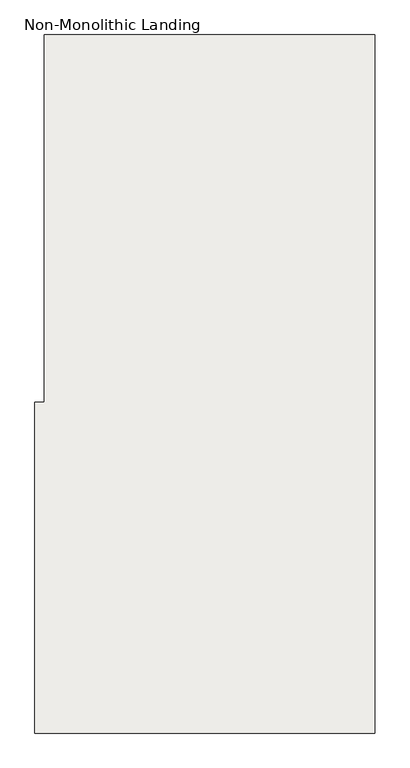
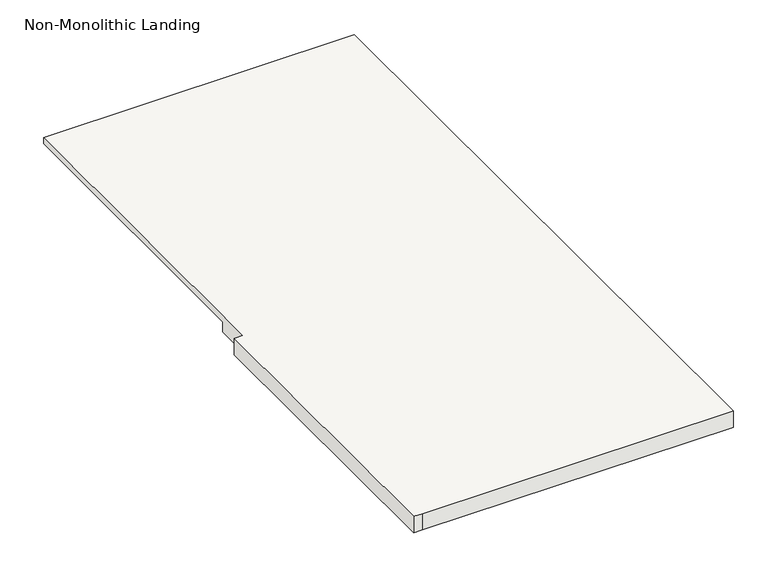
"""IFC4 building model written with IfcOpenShell, lengths in millimetres: slab geometry, Non-Monolithic Landing."""

from ifc_helpers import new_model, si_unit, origin, place, context, project, spatial, faceted_brep, source, transform, mapped, element, save


def non_monolithic_landing_13b6ecfc(model_context):
    return source(origin(), model_context, "Body", "Brep", [
        faceted_brep([(923.4845537, -3822.9544725, 14382.75), (948.8845537, -3822.9544725, 14357.35), (948.8845537, -4737.3544725, 14357.35), (923.4845537, -4737.3544725, 14382.75), (923.4845537, -4838.9544725, 14401.8), (898.0845537, -4838.9544725, 14401.8), (898.0845537, -5753.3544725, 14401.8), (923.4845537, -5753.3544725, 14401.8), (1837.8845537, -5753.3544725, 14401.8), (1837.8845537, -3822.9544725, 14401.8), (923.4845537, -3822.9544725, 14401.8), (948.8845537, -4737.3544725, 14351.0), (948.8845537, -3822.9544725, 14351.0), (1837.8845537, -3822.9544725, 14351.0), (1837.8845537, -5753.3544725, 14351.0), (923.4845537, -5753.3544725, 14351.0), (898.0845537, -5753.3544725, 14351.0), (898.0845537, -4838.9544725, 14351.0), (923.4845537, -4838.9544725, 14351.0), (923.4845537, -4737.3544725, 14351.0)], [[[0, 1, 2, 3]], [[4, 5, 6, 7, 8, 9, 10]], [[11, 12, 13, 14, 15, 16, 17, 18, 19]], [[12, 11, 2, 1]], [[11, 19, 3, 2]], [[4, 10, 0, 3, 19, 18]], [[5, 4, 18, 17]], [[6, 5, 17, 16]], [[7, 6, 16, 15]], [[8, 7, 15, 14]], [[9, 8, 14, 13]], [[10, 9, 13, 12, 1, 0]]]),
    ])


if __name__ == "__main__":
    model = new_model("IFC4")
    model_context = context("Model", 3, world=origin())
    ifc_project = project(units=[si_unit("LENGTHUNIT", "METRE", prefix="MILLI")], contexts=[model_context])
    site = spatial("IfcSite", under=ifc_project)
    building = spatial("IfcBuilding", under=site)
    placement = place(None, origin())
    non_monolithic_landing_shape = non_monolithic_landing_13b6ecfc(model_context)
    element("IfcSlab", 1, ObjectType="Non-Monolithic Landing", at=placement, inside=building, context=model_context, shape_type="MappedRepresentation", body=[
        mapped(non_monolithic_landing_shape, transform((0.0, 0.0, 0.0), x_axis=(1.0, 0.0, 0.0), y_axis=(0.0, 1.0, 0.0), z_axis=(0.0, 0.0, 1.0))),
    ])
    save(model, "model.ifc")
